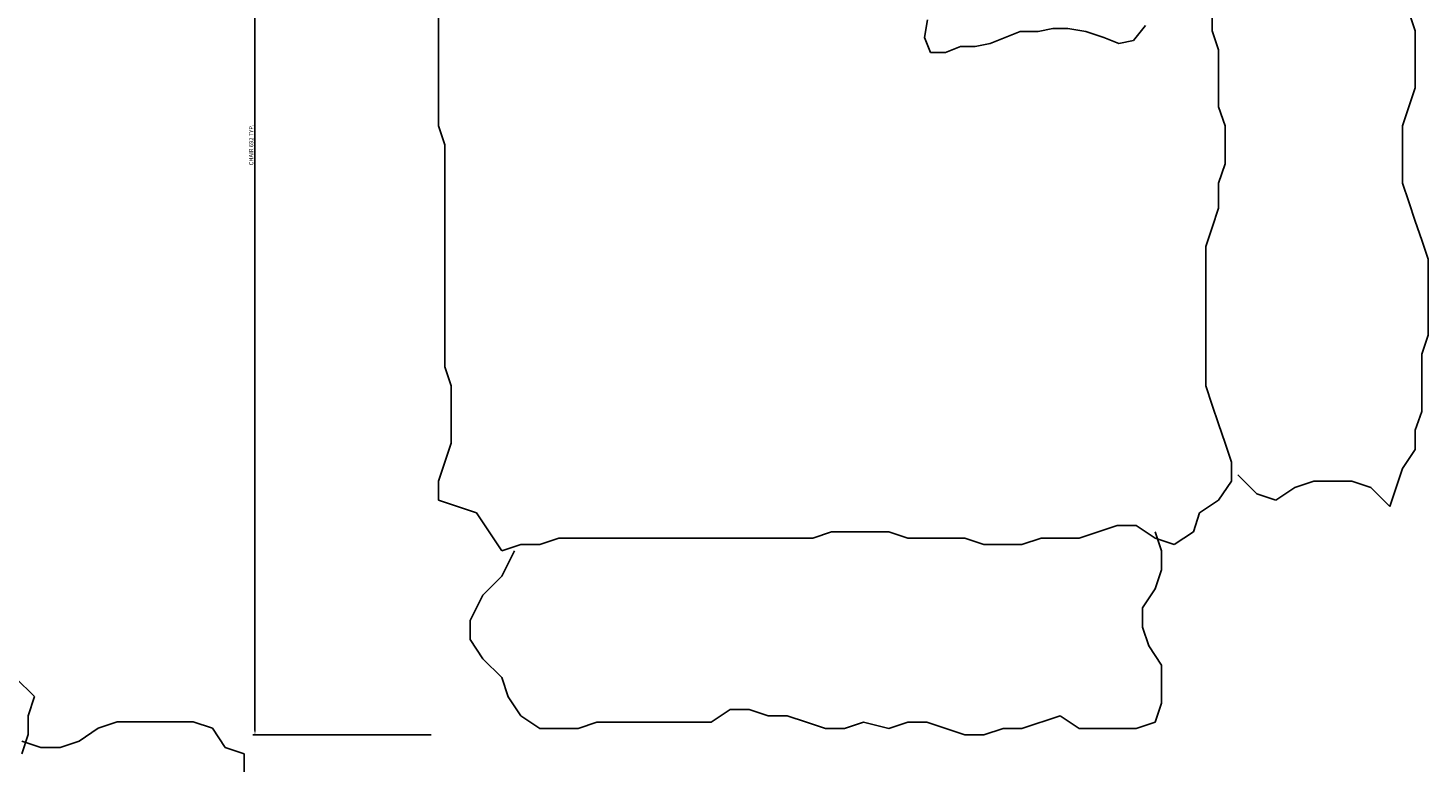
# Model space of a CAD drawing. Units: millimetres. Extents: x -857 to 54106, y -13666 to 13947.
# Tile 24 of 41: x 28540 to 29360, y 10317 to 10747. Entities that reach past the tile are written whole.
import ezdxf

# ---------------------------------------------------------------- set-up
doc = ezdxf.new("R2010")
doc.units = ezdxf.units.MM
doc.layers.add('A-ANNO-DIMS', color=2, linetype='Continuous', lineweight=18)
doc.layers.add('A-FURN', color=21, linetype='Continuous', lineweight=18)
doc.layers.add('TEFRIŞ', color=11, linetype='Continuous')
doc.styles.get("Standard").update_dxf_attribs({"font": 'arial.ttf'})
doc.dimstyles.new('ISO-25', dxfattribs={"dimtxt": 2.5, "dimasz": 2.5, "dimexe": 1.25, "dimexo": 0.625, "dimtad": 1, "dimtxsty": 'Standard', "dimcen": 2.5, "dimadec": 0, "dimazin": 0, "dimtfac": 1, "dimtmove": 0, "dimatfit": 3, "dimfxl": 1, "dimarcsym": 0})

# ---------------------------------------------------------------- blocks, each defined once
blk = doc.blocks.new('25')
at = {"layer": 'TEFRIŞ'}
for p, q in [((-1946.7, -298.17), (-1948.17, -298.66)), ((-1942.27, -298.17), (-1946.7, -298.17)), ((-1940.79, -299.15), (-1942.27, -298.17)), ((-1937.84, -298.17), (-1940.79, -299.15)), ((-1936.37, -298.17), (-1937.84, -298.17)), ((-1934.89, -297.68), (-1936.37, -298.17)), ((-1933.42, -297.68), (-1934.89, -297.68)), ((-1931.94, -298.17), (-1933.42, -297.68)), ((-1930.46, -298.66), (-1931.94, -298.17)), ((-1927.51, -298.17), (-1928.99, -298.66)), ((-1925.54, -298.66), (-1927.51, -298.17)), ((-1924.07, -298.17), (-1925.54, -298.66)), ((-1922.59, -298.17), (-1924.07, -298.17)), ((-1921.12, -298.66), (-1922.59, -298.17)), ((-1903.41, -298.17), (-1904.88, -298.66)), ((-1900.45, -298.17), (-1903.41, -298.17)), ((-1898.98, -299.15), (-1900.45, -298.17)), ((-1948.17, -298.66), (-1948.67, -300.14)), ((-1928.99, -298.66), (-1930.46, -298.66)), ((-1919.64, -299.15), (-1921.12, -298.66)), ((-1918.16, -299.15), (-1919.64, -299.15)), ((-1916.69, -299.64), (-1918.16, -299.15)), ((-1915.21, -299.64), (-1916.69, -299.64)), ((-1913.74, -298.66), (-1915.21, -299.64)), ((-1904.88, -298.66), (-1913.74, -298.66)), ((-1897.99, -300.63), (-1898.98, -299.15)), ((-1948.67, -300.14), (-1948.67, -303.09)), ((-1897.5, -302.11), (-1897.99, -300.63)), ((-1896.03, -303.58), (-1897.5, -302.11)), ((-1948.67, -303.09), (-1947.68, -304.57)), ((-1895.04, -305.06), (-1896.03, -303.58)), ((-1947.68, -304.57), (-1947.19, -306.04)), ((-1895.04, -306.54), (-1895.04, -305.06)), ((-1947.19, -306.04), (-1947.19, -307.52)), ((-1896.03, -308.51), (-1895.04, -306.54)), ((-1947.19, -307.52), (-1948.17, -309)), ((-1948.17, -309), (-1948.67, -310.47)), ((-1897.5, -309.98), (-1896.03, -308.51)), ((-1948.67, -310.47), (-1948.67, -311.95)), ((-1898.49, -311.95), (-1897.5, -309.98)), ((-1949.65, -312.44), (-1951.13, -313.43)), ((-1948.17, -312.94), (-1949.65, -312.44)), ((-1948.67, -311.95), (-1948.17, -313.43)), ((-1937.84, -312.44), (-1939.32, -312.94)), ((-1934.89, -312.44), (-1937.84, -312.44)), ((-1933.42, -312.94), (-1934.89, -312.44)), ((-1900.45, -312.44), (-1901.93, -312.94)), ((-1898.98, -312.44), (-1900.45, -312.44)), ((-1897.5, -311.95), (-1898.98, -312.44)), ((-1896.52, -313.43), (-1897.5, -311.95)), ((-1951.13, -313.43), (-1951.62, -314.91)), ((-1946.7, -313.92), (-1948.17, -312.94)), ((-1943.75, -313.43), (-1945.22, -313.92)), ((-1942.27, -312.94), (-1943.75, -313.43)), ((-1939.32, -312.94), (-1942.27, -312.94)), ((-1928.99, -312.94), (-1933.42, -312.94)), ((-1927.51, -313.43), (-1928.99, -312.94)), ((-1923.08, -313.43), (-1927.51, -313.43)), ((-1921.61, -312.94), (-1923.08, -313.43)), ((-1901.93, -312.94), (-1921.61, -312.94)), ((-1895.53, -314.91), (-1896.52, -313.43)), ((-1945.22, -313.92), (-1946.7, -313.92)), ((-1966.87, -316.87), (-1966.38, -315.4)), ((-1966.38, -315.4), (-1964.9, -316.87)), ((-1959, -316.87), (-1957.52, -315.89)), ((-1957.52, -315.89), (-1956.05, -316.38)), ((-1953.09, -315.89), (-1954.08, -317.37)), ((-1951.62, -314.91), (-1953.09, -315.89)), ((-1894.06, -315.4), (-1895.53, -314.91)), ((-1892.58, -315.89), (-1894.06, -315.4)), ((-1892.58, -317.37), (-1892.58, -315.89)), ((-1967.36, -318.35), (-1966.87, -316.87)), ((-1964.9, -316.87), (-1963.42, -317.37)), ((-1960.47, -317.37), (-1959, -316.87)), ((-1956.05, -316.38), (-1954.57, -317.86)), ((-1963.42, -317.37), (-1960.47, -317.37)), ((-1954.08, -317.37), (-1954.08, -318.84)), ((-1893.08, -318.84), (-1892.58, -317.37)), ((-1968.34, -319.83), (-1967.36, -318.35)), ((-1954.08, -318.84), (-1953.59, -320.32)), ((-1893.57, -320.32), (-1893.08, -318.84)), ((-1968.34, -321.31), (-1968.34, -319.83)), ((-1968.84, -322.78), (-1968.34, -321.31)), ((-1953.59, -320.32), (-1953.09, -321.8)), ((-1893.57, -324.75), (-1893.57, -320.32)), ((-1953.09, -321.8), (-1952.6, -323.27)), ((-1968.84, -327.21), (-1968.84, -322.78)), ((-1952.6, -323.27), (-1952.11, -324.75)), ((-1952.11, -324.75), (-1952.11, -335.58)), ((-1893.08, -326.23), (-1893.57, -324.75)), ((-1893.08, -343.46), (-1893.08, -326.23)), ((-1969.33, -328.69), (-1968.84, -327.21)), ((-1969.33, -334.6), (-1969.33, -328.69)), ((-1968.84, -336.07), (-1969.33, -334.6)), ((-1968.34, -337.55), (-1968.84, -336.07)), ((-1952.11, -335.58), (-1952.6, -337.06)), ((-1967.85, -339.03), (-1968.34, -337.55)), ((-1952.6, -337.06), (-1953.09, -338.54)), ((-1953.09, -338.54), (-1953.09, -340.5)), ((-1967.36, -340.5), (-1967.85, -339.03)), ((-1967.36, -344.94), (-1967.36, -340.5)), ((-1953.09, -340.5), (-1953.59, -341.98)), ((-1953.59, -341.98), (-1953.59, -344.94)), ((-1892.58, -344.94), (-1893.08, -343.46)), ((-1967.85, -346.41), (-1967.36, -344.94)), ((-1953.59, -344.94), (-1953.09, -346.41)), ((-1892.58, -362.17), (-1892.58, -344.94)), ((-1968.34, -347.89), (-1967.85, -346.41)), ((-1953.09, -346.41), (-1953.09, -350.84)), ((-1968.34, -352.32), (-1968.34, -347.89)), ((-1933.06, -351.09), (-1931.9, -350.63)), ((-1931.9, -350.63), (-1930.74, -350.63)), ((-1930.74, -350.63), (-1930.28, -351.79)), ((-1953.09, -350.84), (-1952.6, -352.32)), ((-1947.43, -352.72), (-1946.5, -351.56)), ((-1946.5, -351.56), (-1945.34, -351.33)), ((-1945.34, -351.33), (-1944.19, -351.79)), ((-1936.54, -351.79), (-1935.38, -351.33)), ((-1935.38, -351.33), (-1934.22, -351.09)), ((-1934.22, -351.09), (-1933.06, -351.09)), ((-1967.85, -353.8), (-1968.34, -352.32)), ((-1952.6, -352.32), (-1952.6, -354.29)), ((-1944.19, -351.79), (-1942.79, -352.25)), ((-1942.79, -352.25), (-1941.4, -352.49)), ((-1941.4, -352.49), (-1940.24, -352.49)), ((-1940.24, -352.49), (-1939.09, -352.25)), ((-1939.09, -352.25), (-1937.69, -352.25)), ((-1937.69, -352.25), (-1936.54, -351.79)), ((-1930.28, -351.79), (-1930.51, -353.18))]:
    blk.add_line(p, q, dxfattribs=at)
blk = doc.blocks.new('26')
at = {"layer": 'TEFRIŞ'}
for p, q in [((-1607.8, -262.65), (-1607.31, -261.17)), ((-1607.31, -261.17), (-1605.84, -261.17)), ((-1609.28, -263.63), (-1607.8, -262.65)), ((-1609.77, -265.11), (-1609.28, -263.63)), ((-1609.77, -271.02), (-1609.77, -265.11)), ((-1609.28, -272.49), (-1609.77, -271.02)), ((-1608.29, -273.97), (-1609.28, -272.49)), ((-1607.8, -275.45), (-1608.29, -273.97)), ((-1607.8, -276.93), (-1607.8, -275.45)), ((-1611.74, -277.42), (-1613.21, -278.89)), ((-1610.26, -277.91), (-1611.74, -277.42)), ((-1608.79, -277.91), (-1610.26, -277.91)), ((-1607.31, -278.4), (-1608.79, -277.91)), ((-1608.29, -278.4), (-1607.8, -276.93))]:
    blk.add_line(p, q, dxfattribs=at)
blk = doc.blocks.new('*D49')
at = {"layer": 'A-ANNO-DIMS', "color": 0, "lineweight": -2, "transparency": 16777216}
for p, q in [((28776.01, 11024.79), (28671.56, 11024.79)), ((28672.81, 11022.29), (28672.81, 10335.12)), ((28776.01, 10332.62), (28671.56, 10332.62))]:
    blk.add_line(p, q, dxfattribs=at)
at = {"layer": 'A-ANNO-DIMS', "color": 0, "transparency": 16777216}
for points in [[(28672.39, 11022.29), (28673.22, 11022.29), (28672.81, 11024.79)], [(28672.39, 10335.12), (28673.22, 10335.12), (28672.81, 10332.62)]]:
    blk.add_solid(points, dxfattribs=at)
at = {"layer": 'Defpoints', "color": 0, "transparency": 16777216}
for p in [(28776.63, 11024.79), (28672.81, 10332.62), (28776.63, 10332.62)]:
    blk.add_point(p, dxfattribs=at)
at = {"layer": 'A-ANNO-DIMS', "color": 0, "transparency": 16777216, "insert": (28670.89, 10678.71), "char_height": 2.5, "attachment_point": 5, "rotation": 90}
blk.add_mtext('CHAIR 692 TYP.', dxfattribs=at)

msp = doc.modelspace()

# ---------------------------------------------------------------- block references
at = {"layer": 'A-FURN', "xscale": 7.559220362162901, "yscale": 7.559220362162901, "zscale": 7.559220362162901}
for name, p, rotation in [('25', (14473.896, 8082.429), 180), ('26', (30640.69, -1828.483), 270)]:
    msp.add_blockref(name, p, dxfattribs=dict(at, rotation=rotation))

# ---------------------------------------------------------------- dimensions: what is measured, and where the dimension line sits
at = {"layer": 'A-ANNO-DIMS'}
dim = msp.add_linear_dim(base=(28672.806, 10332.624), p1=(28776.63, 11024.786), p2=(28776.63, 10332.624), angle=270, text='CHAIR <> TYP.', dimstyle='ISO-25', override={"dimdec": 0, "dimrnd": 0, "dimzin": 0, "dimlunit": 2}, dxfattribs=at)
dim.commit()
dim.dimension.update_dxf_attribs({"geometry": '*D49', "text_midpoint": (28670.888, 10678.705)})

doc.saveas('drawing.dxf')
